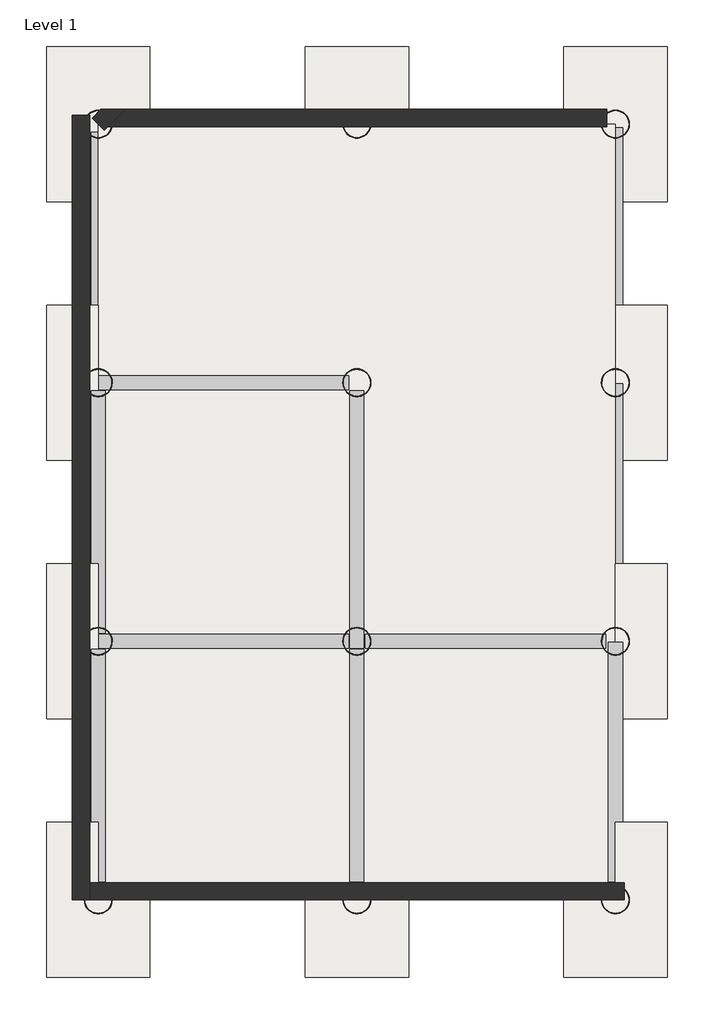
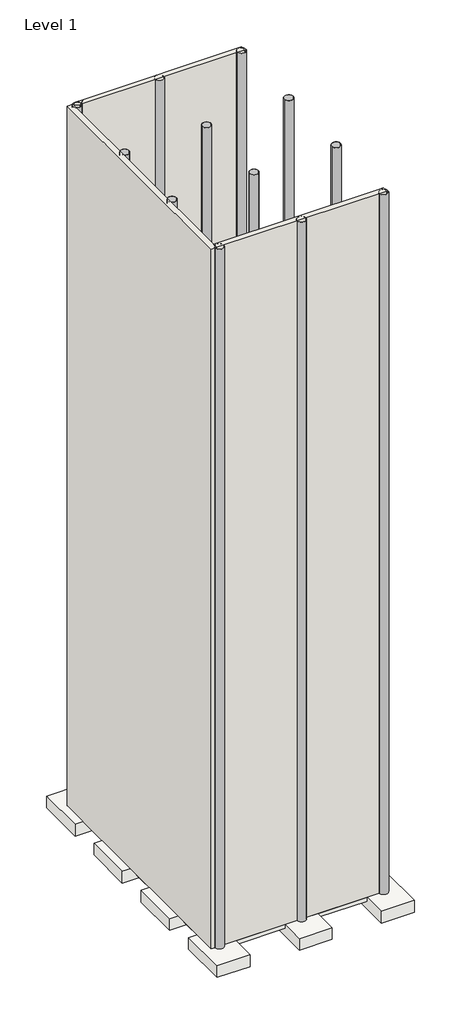
# One storey: 15 beams, 13 slabs, 12 columns, 4 walls.
"""IFC4 building model written with IfcOpenShell, lengths in millimetres."""

from ifc_helpers import new_model, si_unit, frame, origin, place, context, project, spatial, polyline, outline, extrude, faceted_brep, transform, mapped, element, save
from components import ub_universal_beams_ub305x165x40_219eb426, ub_universal_beams_ub305x165x40_d74fc5b0, ub_universal_beams_ub305x165x40_f0dc7efd, ub_universal_beams_ub305x165x40_603755b3, ub_universal_beams_ub305x165x40_59f247e4, ub_universal_beams_ub305x165x40_82a0cad5, ub_universal_beams_ub305x165x40_f6c4464a, ub_universal_beams_ub305x165x40_59e17645, ub_universal_beams_ub305x165x40_3a463868, ub_universal_beams_ub305x165x40_ffb14e35, ub_universal_beams_beam_d94dd637, pipe_column_pipe12std_f9386f83

model = new_model("IFC4")

# Units and contexts
model_context = context("Model", 3, world=origin())
ifc_project = project(units=[si_unit("LENGTHUNIT", "METRE", prefix="MILLI")], contexts=[model_context])

# Site, building, storey
site = spatial("IfcSite", under=ifc_project)
building = spatial("IfcBuilding", under=site)
storey = spatial("IfcBuildingStorey", under=building, Name="Level 1", Elevation=0.0)

# Beams
placement = place(None, origin())
ub_universal_beams_ub305x165x40_shape = ub_universal_beams_ub305x165x40_219eb426(model_context)
element("IfcBeam", 1, ObjectType="UB-Universal Beams : UB305x165x40", at=placement, inside=storey, context=model_context, shape_type="MappedRepresentation", body=[
    mapped(ub_universal_beams_ub305x165x40_shape, transform((13935.1404262, -1814.7314166, -151.7), x_axis=(0.0, 1.0, 0.0), y_axis=(-1.0, 0.0, 0.0), z_axis=(0.0, 0.0, 1.0))),
])
ub_universal_beams_ub305x165x40_2_shape = ub_universal_beams_ub305x165x40_d74fc5b0(model_context)
element("IfcBeam", 2, ObjectType="UB-Universal Beams : UB305x165x40", at=placement, inside=storey, context=model_context, shape_type="MappedRepresentation", body=[
    mapped(ub_universal_beams_ub305x165x40_2_shape, transform((16935.1404262, -1814.7314166, -151.7), x_axis=(0.0, 1.0, 0.0), y_axis=(-1.0, 0.0, 0.0), z_axis=(0.0, 0.0, 1.0))),
])
ub_universal_beams_ub305x165x40_3_shape = ub_universal_beams_ub305x165x40_f0dc7efd(model_context)
element("IfcBeam", 3, ObjectType="UB-Universal Beams : UB305x165x40", at=placement, inside=storey, context=model_context, shape_type="MappedRepresentation", body=[
    mapped(ub_universal_beams_ub305x165x40_3_shape, transform((15435.1404262, -3314.7314166, -151.7), x_axis=(-1.0, 0.0, 0.0), y_axis=(0.0, -1.0, 0.0), z_axis=(0.0, 0.0, 1.0))),
])
element("IfcBeam", 4, ObjectType="UB-Universal Beams : UB305x165x40", at=placement, inside=storey, context=model_context, shape_type="MappedRepresentation", body=[
    mapped(ub_universal_beams_ub305x165x40_3_shape, transform((15435.1404262, -314.7314166, -151.7), x_axis=(-1.0, 0.0, 0.0), y_axis=(0.0, -1.0, 0.0), z_axis=(0.0, 0.0, 1.0))),
])
element("IfcBeam", 5, ObjectType="UB-Universal Beams : UB305x165x40", at=placement, inside=storey, context=model_context, shape_type="MappedRepresentation", body=[
    mapped(ub_universal_beams_ub305x165x40_shape, transform((13935.1404262, 1185.2685834, -151.7), x_axis=(0.0, 1.0, 0.0), y_axis=(-1.0, 0.0, 0.0), z_axis=(0.0, 0.0, 1.0))),
])
ub_universal_beams_ub305x165x40_4_shape = ub_universal_beams_ub305x165x40_603755b3(model_context)
element("IfcBeam", 6, ObjectType="UB-Universal Beams : UB305x165x40", at=placement, inside=storey, context=model_context, shape_type="MappedRepresentation", body=[
    mapped(ub_universal_beams_ub305x165x40_4_shape, transform((15435.1404262, 2685.2685834, -151.7), x_axis=(-1.0, 0.0, 0.0), y_axis=(0.0, -1.0, 0.0), z_axis=(0.0, 0.0, 1.0))),
])
ub_universal_beams_ub305x165x40_5_shape = ub_universal_beams_ub305x165x40_59f247e4(model_context)
element("IfcBeam", 7, ObjectType="UB-Universal Beams : UB305x165x40", at=placement, inside=storey, context=model_context, shape_type="MappedRepresentation", body=[
    mapped(ub_universal_beams_ub305x165x40_5_shape, transform((16935.1404262, 1220.6239224, -151.7), x_axis=(0.0, 1.0, 0.0), y_axis=(-1.0, 0.0, 0.0), z_axis=(0.0, 0.0, 1.0))),
])
ub_universal_beams_ub305x165x40_6_shape = ub_universal_beams_ub305x165x40_82a0cad5(model_context)
element("IfcBeam", 8, ObjectType="UB-Universal Beams : UB305x165x40", at=placement, inside=storey, context=model_context, shape_type="MappedRepresentation", body=[
    mapped(ub_universal_beams_ub305x165x40_6_shape, transform((18435.1404262, -3314.7314166, -151.7), x_axis=(-1.0, 0.0, 0.0), y_axis=(0.0, -1.0, 0.0), z_axis=(0.0, 0.0, 1.0))),
])
element("IfcBeam", 9, ObjectType="UB-Universal Beams : UB305x165x40", at=placement, inside=storey, context=model_context, shape_type="MappedRepresentation", body=[
    mapped(ub_universal_beams_ub305x165x40_6_shape, transform((18435.1404262, -314.7314166, -151.7), x_axis=(-1.0, 0.0, 0.0), y_axis=(0.0, -1.0, 0.0), z_axis=(0.0, 0.0, 1.0))),
])
ub_universal_beams_ub305x165x40_7_shape = ub_universal_beams_ub305x165x40_f6c4464a(model_context)
element("IfcBeam", 10, ObjectType="UB-Universal Beams : UB305x165x40", at=placement, inside=storey, context=model_context, shape_type="MappedRepresentation", body=[
    mapped(ub_universal_beams_ub305x165x40_7_shape, transform((18435.1404262, 2685.2685834, -151.7), x_axis=(-1.0, 0.0, 0.0), y_axis=(0.0, -1.0, 0.0), z_axis=(0.0, 0.0, 1.0))),
])
ub_universal_beams_ub305x165x40_8_shape = ub_universal_beams_ub305x165x40_59e17645(model_context)
element("IfcBeam", 11, ObjectType="UB-Universal Beams : UB305x165x40", at=placement, inside=storey, context=model_context, shape_type="MappedRepresentation", body=[
    mapped(ub_universal_beams_ub305x165x40_8_shape, transform((19935.1404262, -1814.7314166, -151.7), x_axis=(0.0, 1.0, 0.0), y_axis=(-1.0, 0.0, 0.0), z_axis=(0.0, 0.0, 1.0))),
])
ub_universal_beams_ub305x165x40_9_shape = ub_universal_beams_ub305x165x40_3a463868(model_context)
element("IfcBeam", 12, ObjectType="UB-Universal Beams : UB305x165x40", at=placement, inside=storey, context=model_context, shape_type="MappedRepresentation", body=[
    mapped(ub_universal_beams_ub305x165x40_9_shape, transform((19935.1404262, 1220.6239224, -151.7), x_axis=(0.0, 1.0, 0.0), y_axis=(-1.0, 0.0, 0.0), z_axis=(0.0, 0.0, 1.0))),
])
ub_universal_beams_ub305x165x40_10_shape = ub_universal_beams_ub305x165x40_ffb14e35(model_context)
element("IfcBeam", 13, ObjectType="UB-Universal Beams : UB305x165x40", at=placement, inside=storey, context=model_context, shape_type="MappedRepresentation", body=[
    mapped(ub_universal_beams_ub305x165x40_10_shape, transform((13935.1404262, -4764.7314166, -151.7), x_axis=(0.0, 1.0, 0.0), y_axis=(-1.0, 0.0, 0.0), z_axis=(0.0, 0.0, 1.0))),
])
element("IfcBeam", 14, ObjectType="UB-Universal Beams : UB305x165x40", at=placement, inside=storey, context=model_context, shape_type="MappedRepresentation", body=[
    mapped(ub_universal_beams_ub305x165x40_10_shape, transform((16935.1404262, -4764.7314166, -151.7), x_axis=(0.0, 1.0, 0.0), y_axis=(-1.0, 0.0, 0.0), z_axis=(0.0, 0.0, 1.0))),
])
ub_universal_beams_beam_shape = ub_universal_beams_beam_d94dd637(model_context)
element("IfcBeam", 15, ObjectType="UB-Universal Beams : beam", at=placement, inside=storey, context=model_context, shape_type="MappedRepresentation", body=[
    mapped(ub_universal_beams_beam_shape, transform((19935.1404262, -4764.7314166, -151.7), x_axis=(0.0, 1.0, 0.0), y_axis=(-1.0, 0.0, 0.0), z_axis=(0.0, 0.0, 1.0))),
])

# Columns
pipe_column_pipe12std_shape = pipe_column_pipe12std_f9386f83(model_context)
element("IfcColumn", 16, ObjectType="Pipe Column : Pipe12STD", at=placement, inside=storey, context=model_context, shape_type="MappedRepresentation", body=[
    mapped(pipe_column_pipe12std_shape, transform((13935.1404262, -6314.7314166, 0.0), x_axis=(-1.0, 0.0, 0.0), y_axis=(0.0, -1.0, 0.0), z_axis=(0.0, 0.0, 1.0))),
])
element("IfcColumn", 17, ObjectType="Pipe Column : Pipe12STD", at=placement, inside=storey, context=model_context, shape_type="MappedRepresentation", body=[
    mapped(pipe_column_pipe12std_shape, transform((16935.1404262, -6314.7314166, 0.0), x_axis=(-1.0, 0.0, 0.0), y_axis=(0.0, -1.0, 0.0), z_axis=(0.0, 0.0, 1.0))),
])
element("IfcColumn", 18, ObjectType="Pipe Column : Pipe12STD", at=placement, inside=storey, context=model_context, shape_type="MappedRepresentation", body=[
    mapped(pipe_column_pipe12std_shape, transform((19935.1404262, -6314.7314166, 0.0), x_axis=(-1.0, 0.0, 0.0), y_axis=(0.0, -1.0, 0.0), z_axis=(0.0, 0.0, 1.0))),
])
element("IfcColumn", 19, ObjectType="Pipe Column : Pipe12STD", at=placement, inside=storey, context=model_context, shape_type="MappedRepresentation", body=[
    mapped(pipe_column_pipe12std_shape, transform((13935.1404262, -3314.7314166, 0.0), x_axis=(-1.0, 0.0, 0.0), y_axis=(0.0, -1.0, 0.0), z_axis=(0.0, 0.0, 1.0))),
])
element("IfcColumn", 20, ObjectType="Pipe Column : Pipe12STD", at=placement, inside=storey, context=model_context, shape_type="MappedRepresentation", body=[
    mapped(pipe_column_pipe12std_shape, transform((13935.1404262, -314.7314166, 0.0), x_axis=(-1.0, 0.0, 0.0), y_axis=(0.0, -1.0, 0.0), z_axis=(0.0, 0.0, 1.0))),
])
element("IfcColumn", 21, ObjectType="Pipe Column : Pipe12STD", at=placement, inside=storey, context=model_context, shape_type="MappedRepresentation", body=[
    mapped(pipe_column_pipe12std_shape, transform((13935.1404262, 2685.2685834, 0.0), x_axis=(-1.0, 0.0, 0.0), y_axis=(0.0, -1.0, 0.0), z_axis=(0.0, 0.0, 1.0))),
])
element("IfcColumn", 22, ObjectType="Pipe Column : Pipe12STD", at=placement, inside=storey, context=model_context, shape_type="MappedRepresentation", body=[
    mapped(pipe_column_pipe12std_shape, transform((16935.1404262, -3314.7314166, 0.0), x_axis=(-1.0, 0.0, 0.0), y_axis=(0.0, -1.0, 0.0), z_axis=(0.0, 0.0, 1.0))),
])
element("IfcColumn", 23, ObjectType="Pipe Column : Pipe12STD", at=placement, inside=storey, context=model_context, shape_type="MappedRepresentation", body=[
    mapped(pipe_column_pipe12std_shape, transform((19935.1404262, -3314.7314166, 0.0), x_axis=(-1.0, 0.0, 0.0), y_axis=(0.0, -1.0, 0.0), z_axis=(0.0, 0.0, 1.0))),
])
element("IfcColumn", 24, ObjectType="Pipe Column : Pipe12STD", at=placement, inside=storey, context=model_context, shape_type="MappedRepresentation", body=[
    mapped(pipe_column_pipe12std_shape, transform((16935.1404262, -314.7314166, 0.0), x_axis=(-1.0, 0.0, 0.0), y_axis=(0.0, -1.0, 0.0), z_axis=(0.0, 0.0, 1.0))),
])
element("IfcColumn", 25, ObjectType="Pipe Column : Pipe12STD", at=placement, inside=storey, context=model_context, shape_type="MappedRepresentation", body=[
    mapped(pipe_column_pipe12std_shape, transform((19935.1404262, -314.7314166, 0.0), x_axis=(-1.0, 0.0, 0.0), y_axis=(0.0, -1.0, 0.0), z_axis=(0.0, 0.0, 1.0))),
])
element("IfcColumn", 26, ObjectType="Pipe Column : Pipe12STD", at=placement, inside=storey, context=model_context, shape_type="MappedRepresentation", body=[
    mapped(pipe_column_pipe12std_shape, transform((16935.1404262, 2685.2685834, 0.0), x_axis=(-1.0, 0.0, 0.0), y_axis=(0.0, -1.0, 0.0), z_axis=(0.0, 0.0, 1.0))),
])
element("IfcColumn", 27, ObjectType="Pipe Column : Pipe12STD", at=placement, inside=storey, context=model_context, shape_type="MappedRepresentation", body=[
    mapped(pipe_column_pipe12std_shape, transform((19935.1404262, 2685.2685834, 0.0), x_axis=(-1.0, 0.0, 0.0), y_axis=(0.0, -1.0, 0.0), z_axis=(0.0, 0.0, 1.0))),
])

# Slabs
element("IfcSlab", 28, ObjectType="150mm Foundation Slab", at=placement, inside=storey, context=model_context, shape_type="Brep", body=[
    faceted_brep([(13935.1404262, -6314.7314166, -150.0), (13935.1404262, -5414.7314166, -150.0), (13935.1404262, -4214.7314166, -150.0), (13935.1404262, -2414.7314166, -150.0), (13935.1404262, -1214.7314166, -150.0), (13935.1404262, 585.2685834, -150.0), (13935.1404262, 1785.2685834, -150.0), (13935.1404262, 2685.2685834, -150.0), (14535.1404262, 2685.2685834, -150.0), (16335.1404262, 2685.2685834, -150.0), (17535.1404262, 2685.2685834, -150.0), (19335.1404262, 2685.2685834, -150.0), (19935.1404262, 2685.2685834, -150.0), (19935.1404262, 1785.2685834, -150.0), (19935.1404262, 585.2685834, -150.0), (19935.1404262, -1214.7314166, -150.0), (19935.1404262, -2414.7314166, -150.0), (19935.1404262, -4214.7314166, -150.0), (19935.1404262, -5414.7314166, -150.0), (19935.1404262, -6314.7314166, -150.0), (19335.1404262, -6314.7314166, -150.0), (17535.1404262, -6314.7314166, -150.0), (16335.1404262, -6314.7314166, -150.0), (14535.1404262, -6314.7314166, -150.0), (13935.1404262, -6314.7314166, 0.0), (14535.1404262, -6314.7314166, 0.0), (16335.1404262, -6314.7314166, 0.0), (17535.1404262, -6314.7314166, 0.0), (19335.1404262, -6314.7314166, 0.0), (19935.1404262, -6314.7314166, 0.0), (19935.1404262, -5414.7314166, 0.0), (19935.1404262, -4214.7314166, 0.0), (19935.1404262, -2414.7314166, 0.0), (19935.1404262, -1214.7314166, 0.0), (19935.1404262, 585.2685834, 0.0), (19935.1404262, 1785.2685834, 0.0), (19935.1404262, 2685.2685834, 0.0), (19335.1404262, 2685.2685834, 0.0), (17535.1404262, 2685.2685834, 0.0), (16335.1404262, 2685.2685834, 0.0), (14535.1404262, 2685.2685834, 0.0), (13935.1404262, 2685.2685834, 0.0), (13935.1404262, 1785.2685834, 0.0), (13935.1404262, 585.2685834, 0.0), (13935.1404262, -1214.7314166, 0.0), (13935.1404262, -2414.7314166, 0.0), (13935.1404262, -4214.7314166, 0.0), (13935.1404262, -5414.7314166, 0.0)], [[[0, 1, 2, 3, 4, 5, 6, 7, 8, 9, 10, 11, 12, 13, 14, 15, 16, 17, 18, 19, 20, 21, 22, 23]], [[24, 25, 26, 27, 28, 29, 30, 31, 32, 33, 34, 35, 36, 37, 38, 39, 40, 41, 42, 43, 44, 45, 46, 47]], [[7, 6, 5, 4, 3, 2, 1, 0, 24, 47, 46, 45, 44, 43, 42, 41]], [[12, 11, 10, 9, 8, 7, 41, 40, 39, 38, 37, 36]], [[19, 18, 17, 16, 15, 14, 13, 12, 36, 35, 34, 33, 32, 31, 30, 29]], [[0, 23, 22, 21, 20, 19, 29, 28, 27, 26, 25, 24]]]),
])
element("IfcSlab", 29, ObjectType="M_Footing-Rectangular : 1800 x 1200 x 450mm", at=placement, inside=storey, context=model_context, shape_type="Brep", body=[
    faceted_brep([(13335.1404262, -7214.7314166, 0.0), (14535.1404262, -7214.7314166, 0.0), (14535.1404262, -6314.7314166, 0.0), (13935.1404262, -6314.7314166, 0.0), (13935.1404262, -5414.7314166, 0.0), (13335.1404262, -5414.7314166, 0.0), (13335.1404262, -7214.7314166, -450.0), (13335.1404262, -5414.7314166, -450.0), (14535.1404262, -5414.7314166, -450.0), (14535.1404262, -7214.7314166, -450.0), (14535.1404262, -5414.7314166, -150.0), (14535.1404262, -6314.7314166, -150.0), (13935.1404262, -5414.7314166, -150.0), (13935.1404262, -6314.7314166, -150.0)], [[[0, 1, 2, 3, 4, 5]], [[6, 7, 8, 9]], [[1, 0, 6, 9]], [[9, 8, 10, 11, 2, 1]], [[8, 7, 5, 4, 12, 10]], [[0, 5, 7, 6]], [[13, 11, 10, 12]], [[3, 13, 12, 4]], [[13, 3, 2, 11]]]),
])
element("IfcSlab", 30, ObjectType="M_Footing-Rectangular : 1800 x 1200 x 450mm", at=placement, inside=storey, context=model_context, shape_type="SweptSolid", body=[
    extrude(outline(polyline([(-5414.7314166, -450.0), (-7214.7314166, -450.0), (-7214.7314166, 0.0), (-6314.7314166, 0.0), (-6314.7314166, -150.0), (-5414.7314166, -150.0), (-5414.7314166, -450.0)])), frame((16335.1404262, 0.0, 0.0), z_axis=(1.0, 0.0, 0.0), x_axis=(0.0, 1.0, 0.0)), (0.0, 0.0, 1.0), 1200.0),
])
element("IfcSlab", 31, ObjectType="M_Footing-Rectangular : 1800 x 1200 x 450mm", at=placement, inside=storey, context=model_context, shape_type="Brep", body=[
    faceted_brep([(19335.1404262, -7214.7314166, 0.0), (20535.1404262, -7214.7314166, 0.0), (20535.1404262, -5414.7314166, 0.0), (19935.1404262, -5414.7314166, 0.0), (19935.1404262, -6314.7314166, 0.0), (19335.1404262, -6314.7314166, 0.0), (19335.1404262, -7214.7314166, -450.0), (19335.1404262, -5414.7314166, -450.0), (20535.1404262, -5414.7314166, -450.0), (20535.1404262, -7214.7314166, -450.0), (19335.1404262, -5414.7314166, -150.0), (19935.1404262, -5414.7314166, -150.0), (19335.1404262, -6314.7314166, -150.0), (19935.1404262, -6314.7314166, -150.0)], [[[0, 1, 2, 3, 4, 5]], [[6, 7, 8, 9]], [[1, 0, 6, 9]], [[2, 1, 9, 8]], [[8, 7, 10, 11, 3, 2]], [[7, 6, 0, 5, 12, 10]], [[12, 13, 11, 10]], [[13, 4, 3, 11]], [[4, 13, 12, 5]]]),
])
element("IfcSlab", 32, ObjectType="M_Footing-Rectangular : 1800 x 1200 x 450mm", at=placement, inside=storey, context=model_context, shape_type="SweptSolid", body=[
    extrude(outline(polyline([(-450.0, 13335.1404262), (-450.0, 14535.1404262), (-150.0, 14535.1404262), (-150.0, 13935.1404262), (0.0, 13935.1404262), (0.0, 13335.1404262), (-450.0, 13335.1404262)])), frame((0.0, -4214.7314166, 0.0), z_axis=(0.0, 1.0, 0.0), x_axis=(0.0, 0.0, 1.0)), (0.0, 0.0, 1.0), 1800.0),
])
element("IfcSlab", 33, ObjectType="M_Footing-Rectangular : 1800 x 1200 x 450mm", at=placement, inside=storey, context=model_context, shape_type="SweptSolid", body=[
    extrude(outline(polyline([(-450.0, 13335.1404262), (-450.0, 14535.1404262), (-150.0, 14535.1404262), (-150.0, 13935.1404262), (0.0, 13935.1404262), (0.0, 13335.1404262), (-450.0, 13335.1404262)])), frame((0.0, -1214.7314166, 0.0), z_axis=(0.0, 1.0, 0.0), x_axis=(0.0, 0.0, 1.0)), (0.0, 0.0, 1.0), 1800.0),
])
element("IfcSlab", 34, ObjectType="M_Footing-Rectangular : 1800 x 1200 x 450mm", at=placement, inside=storey, context=model_context, shape_type="Brep", body=[
    faceted_brep([(14535.1404262, 3585.2685834, 0.0), (13335.1404262, 3585.2685834, 0.0), (13335.1404262, 1785.2685834, 0.0), (13935.1404262, 1785.2685834, 0.0), (13935.1404262, 2685.2685834, 0.0), (14535.1404262, 2685.2685834, 0.0), (13335.1404262, 1785.2685834, -450.0), (13335.1404262, 3585.2685834, -450.0), (14535.1404262, 3585.2685834, -450.0), (14535.1404262, 1785.2685834, -450.0), (14535.1404262, 1785.2685834, -150.0), (13935.1404262, 1785.2685834, -150.0), (14535.1404262, 2685.2685834, -150.0), (13935.1404262, 2685.2685834, -150.0)], [[[0, 1, 2, 3, 4, 5]], [[6, 7, 8, 9]], [[6, 9, 10, 11, 3, 2]], [[9, 8, 0, 5, 12, 10]], [[1, 0, 8, 7]], [[2, 1, 7, 6]], [[12, 13, 11, 10]], [[13, 4, 3, 11]], [[4, 13, 12, 5]]]),
])
element("IfcSlab", 35, ObjectType="M_Footing-Rectangular : 1800 x 1200 x 450mm", at=placement, inside=storey, context=model_context, shape_type="SweptSolid", body=[
    extrude(outline(polyline([(16335.1404262, -4214.7314166), (16335.1404262, -2414.7314166), (17535.1404262, -2414.7314166), (17535.1404262, -4214.7314166), (16335.1404262, -4214.7314166)])), frame((0.0, 0.0, -450.0), z_axis=(0.0, 0.0, 1.0), x_axis=(1.0, 0.0, 0.0)), (0.0, 0.0, 1.0), 300.0),
])
element("IfcSlab", 36, ObjectType="M_Footing-Rectangular : 1800 x 1200 x 450mm", at=placement, inside=storey, context=model_context, shape_type="SweptSolid", body=[
    extrude(outline(polyline([(-450.0, 19335.1404262), (-450.0, 20535.1404262), (0.0, 20535.1404262), (0.0, 19935.1404262), (-150.0, 19935.1404262), (-150.0, 19335.1404262), (-450.0, 19335.1404262)])), frame((0.0, -4214.7314166, 0.0), z_axis=(0.0, 1.0, 0.0), x_axis=(0.0, 0.0, 1.0)), (0.0, 0.0, 1.0), 1800.0),
])
element("IfcSlab", 37, ObjectType="M_Footing-Rectangular : 1800 x 1200 x 450mm", at=placement, inside=storey, context=model_context, shape_type="SweptSolid", body=[
    extrude(outline(polyline([(16335.1404262, -1214.7314166), (16335.1404262, 585.2685834), (17535.1404262, 585.2685834), (17535.1404262, -1214.7314166), (16335.1404262, -1214.7314166)])), frame((0.0, 0.0, -450.0), z_axis=(0.0, 0.0, 1.0), x_axis=(1.0, 0.0, 0.0)), (0.0, 0.0, 1.0), 300.0),
])
element("IfcSlab", 38, ObjectType="M_Footing-Rectangular : 1800 x 1200 x 450mm", at=placement, inside=storey, context=model_context, shape_type="SweptSolid", body=[
    extrude(outline(polyline([(-450.0, 19335.1404262), (-450.0, 20535.1404262), (0.0, 20535.1404262), (0.0, 19935.1404262), (-150.0, 19935.1404262), (-150.0, 19335.1404262), (-450.0, 19335.1404262)])), frame((0.0, -1214.7314166, 0.0), z_axis=(0.0, 1.0, 0.0), x_axis=(0.0, 0.0, 1.0)), (0.0, 0.0, 1.0), 1800.0),
])
element("IfcSlab", 39, ObjectType="M_Footing-Rectangular : 1800 x 1200 x 450mm", at=placement, inside=storey, context=model_context, shape_type="SweptSolid", body=[
    extrude(outline(polyline([(3585.2685834, -450.0), (1785.2685834, -450.0), (1785.2685834, -150.0), (2685.2685834, -150.0), (2685.2685834, 0.0), (3585.2685834, 0.0), (3585.2685834, -450.0)])), frame((16335.1404262, 0.0, 0.0), z_axis=(1.0, 0.0, 0.0), x_axis=(0.0, 1.0, 0.0)), (0.0, 0.0, 1.0), 1200.0),
])
element("IfcSlab", 40, ObjectType="M_Footing-Rectangular : 1800 x 1200 x 450mm", at=placement, inside=storey, context=model_context, shape_type="Brep", body=[
    faceted_brep([(20535.1404262, 1785.2685834, 0.0), (20535.1404262, 3585.2685834, 0.0), (19335.1404262, 3585.2685834, 0.0), (19335.1404262, 2685.2685834, 0.0), (19935.1404262, 2685.2685834, 0.0), (19935.1404262, 1785.2685834, 0.0), (19335.1404262, 1785.2685834, -450.0), (19335.1404262, 3585.2685834, -450.0), (20535.1404262, 3585.2685834, -450.0), (20535.1404262, 1785.2685834, -450.0), (19935.1404262, 1785.2685834, -150.0), (19335.1404262, 1785.2685834, -150.0), (19335.1404262, 2685.2685834, -150.0), (19935.1404262, 2685.2685834, -150.0)], [[[0, 1, 2, 3, 4, 5]], [[6, 7, 8, 9]], [[6, 9, 0, 5, 10, 11]], [[1, 0, 9, 8]], [[2, 1, 8, 7]], [[7, 6, 11, 12, 3, 2]], [[10, 13, 12, 11]], [[13, 4, 3, 12]], [[4, 13, 10, 5]]]),
])

# Walls
element("IfcWall", 41, ObjectType="Generic - 200mm", at=placement, inside=storey, context=model_context, shape_type="Brep", body=[
    faceted_brep([(14005.8511043, 2614.5579052, 0.0), (14047.2724606, 2655.9792615, 0.0), (14247.2724606, 2855.9792615, 0.0), (14247.2724606, 2855.9792615, 27000.0), (14047.2724606, 2655.9792615, 27000.0), (14005.8511043, 2614.5579052, 27000.0), (13864.4297481, 2755.9792615, 0.0), (13864.4297481, 2755.9792615, 27000.0), (13964.4297481, 2855.9792615, 27000.0), (13964.4297481, 2855.9792615, 0.0)], [[[0, 1, 2, 3, 4, 5]], [[6, 7, 8, 9]], [[2, 1, 0, 6, 9]], [[5, 4, 3, 8, 7]], [[0, 5, 7, 6]], [[3, 2, 9, 8]]]),
])
element("IfcWall", 42, ObjectType="Generic - 200mm", at=placement, inside=storey, context=model_context, shape_type="Brep", body=[
    faceted_brep([(14047.2724606, 2655.9792615, 0.0), (19835.1404262, 2655.9792615, 0.0), (19835.1404262, 2655.9792615, 3000.0), (20035.1404262, 2655.9792615, 3000.0), (20035.1404262, 2655.9792615, 6000.0), (20035.1404262, 2655.9792615, 9000.0), (20035.1404262, 2655.9792615, 12000.0), (20035.1404262, 2655.9792615, 15000.0), (20035.1404262, 2655.9792615, 18000.0), (20035.1404262, 2655.9792615, 21000.0), (20035.1404262, 2655.9792615, 24000.0), (20035.1404262, 2655.9792615, 27000.0), (19835.1404262, 2655.9792615, 27000.0), (14047.2724606, 2655.9792615, 27000.0), (14247.2724606, 2855.9792615, 0.0), (14247.2724606, 2855.9792615, 27000.0), (20035.1404262, 2855.9792615, 27000.0), (20035.1404262, 2855.9792615, 3000.0), (19835.1404262, 2855.9792615, 3000.0), (19835.1404262, 2855.9792615, 0.0)], [[[0, 1, 2, 3, 4, 5, 6, 7, 8, 9, 10, 11, 12, 13]], [[14, 15, 16, 17, 18, 19]], [[1, 0, 14, 19]], [[13, 12, 11, 16, 15]], [[17, 3, 2, 18]], [[2, 1, 19, 18]], [[3, 17, 16, 11, 10, 9, 8, 7, 6, 5, 4]], [[0, 13, 15, 14]]]),
])
element("IfcWall", 43, ObjectType="Generic - 200mm", at=placement, inside=storey, context=model_context, shape_type="Brep", body=[
    faceted_brep([(20035.1404262, -6114.7314166, 27000.0), (20035.1404262, -6114.7314166, 24000.0), (20035.1404262, -6114.7314166, 21000.0), (20035.1404262, -6114.7314166, 18000.0), (20035.1404262, -6114.7314166, 15000.0), (20035.1404262, -6114.7314166, 12000.0), (20035.1404262, -6114.7314166, 9000.0), (20035.1404262, -6114.7314166, 6000.0), (20035.1404262, -6114.7314166, 3000.0), (20035.1404262, -6114.7314166, 0.0), (19835.1404262, -6114.7314166, 0.0), (13835.1404262, -6114.7314166, 0.0), (13835.1404262, -6114.7314166, 27000.0), (19835.1404262, -6114.7314166, 27000.0), (20035.1404262, -6314.7314166, 0.0), (20035.1404262, -6314.7314166, 27000.0), (13835.1404262, -6314.7314166, 27000.0), (13835.1404262, -6314.7314166, 0.0)], [[[0, 1, 2, 3, 4, 5, 6, 7, 8, 9, 10, 11, 12, 13]], [[14, 15, 16, 17]], [[11, 10, 9, 14, 17]], [[0, 13, 12, 16, 15]], [[0, 15, 14, 9, 8, 7, 6, 5, 4, 3, 2, 1]], [[12, 11, 17, 16]]]),
])
element("IfcWall", 44, ObjectType="Generic - 200mm", at=placement, inside=storey, context=model_context, shape_type="Brep", body=[
    faceted_brep([(13835.1404262, -6314.7314166, 0.0), (13835.1404262, -6114.7314166, 0.0), (13835.1404262, 2785.2685834, 0.0), (13835.1404262, 2785.2685834, 27000.0), (13835.1404262, -6114.7314166, 27000.0), (13835.1404262, -6314.7314166, 27000.0), (13635.1404262, -6314.7314166, 0.0), (13635.1404262, -6314.7314166, 27000.0), (13635.1404262, 2785.2685834, 27000.0), (13635.1404262, 2785.2685834, 0.0)], [[[0, 1, 2, 3, 4, 5]], [[6, 7, 8, 9]], [[2, 1, 0, 6, 9]], [[3, 2, 9, 8]], [[5, 4, 3, 8, 7]], [[0, 5, 7, 6]]]),
])

save(model, "model.ifc")

# Revit data of these elements
# Grids (mm)
#   "1": line (7751.128, -6314.731) -> (24761.391, -6314.731)
#   "2": line (13935.14, 6118.893) -> (13935.14, -6314.731)
#   "3": line (7751.128, -3314.731) -> (24761.391, -3314.731)
#   "4": line (7751.128, -314.731) -> (24761.391, -314.731)
#   "5": line (7751.128, 2685.269) -> (24761.391, 2685.269)
#   "6": line (16935.14, 6118.893) -> (16935.14, -6314.731)
#   "7": line (19935.14, 6118.893) -> (19935.14, -6314.731)
#   "8": line (7751.128, -6314.731) -> (24761.391, -6314.731)
#   "9": line (7751.128, -3314.731) -> (24761.391, -3314.731)
#   "10": line (7751.128, -314.731) -> (24761.391, -314.731)
#   "11": line (7751.128, 2685.269) -> (24761.391, 2685.269)
#   "12": line (7751.128, -6314.731) -> (24761.391, -6314.731)
#   "13": line (7751.128, -3314.731) -> (24761.391, -3314.731)
#   "14": line (7751.128, -314.731) -> (24761.391, -314.731)
#   "15": line (7751.128, 2685.269) -> (24761.391, 2685.269)
#   "16": line (7751.128, -6314.731) -> (24761.391, -6314.731)
#   "17": line (7751.128, -3314.731) -> (24761.391, -3314.731)
#   "18": line (7751.128, -314.731) -> (24761.391, -314.731)
#   "19": line (7751.128, 2685.269) -> (24761.391, 2685.269)
#   "20": line (7751.128, -6314.731) -> (24761.391, -6314.731)
#   "21": line (7751.128, -3314.731) -> (24761.391, -3314.731)
#   "22": line (7751.128, -314.731) -> (24761.391, -314.731)
#   "23": line (7751.128, 2685.269) -> (24761.391, 2685.269)
#   "24": line (7751.128, -6314.731) -> (24761.391, -6314.731)
#   "25": line (7751.128, -3314.731) -> (24761.391, -3314.731)
#   "26": line (7751.128, -314.731) -> (24761.391, -314.731)
#   "27": line (7751.128, 2685.269) -> (24761.391, 2685.269)
#   "28": line (7751.128, -6314.731) -> (24761.391, -6314.731)
#   "29": line (7751.128, -3314.731) -> (24761.391, -3314.731)
#   "30": line (7751.128, -314.731) -> (24761.391, -314.731)
#   "31": line (7751.128, 2685.269) -> (24761.391, 2685.269)
#   "32": line (7751.128, -6314.731) -> (24761.391, -6314.731)
#   "33": line (7751.128, -3314.731) -> (24761.391, -3314.731)
#   "34": line (7751.128, -314.731) -> (24761.391, -314.731)
#   "35": line (7751.128, 2685.269) -> (24761.391, 2685.269)
#   "36": line (7751.128, -6314.731) -> (24761.391, -6314.731)
#   "37": line (7751.128, -3314.731) -> (24761.391, -3314.731)
#   "38": line (7751.128, -314.731) -> (24761.391, -314.731)
#   "39": line (7751.128, 2685.269) -> (24761.391, 2685.269)
#   "40": line (7751.128, -6314.731) -> (24761.391, -6314.731)
#   "41": line (7751.128, -3314.731) -> (24761.391, -3314.731)
#   "42": line (7751.128, -314.731) -> (24761.391, -314.731)
#   "43": line (7751.128, 2685.269) -> (24761.391, 2685.269)
# Type "UB-Universal Beams : UB305x165x40"
#   Section Name Key = "UB305X165X40"
#   Width = 16.5 cm
#   Web Thickness = 0.6 cm
#   Web Fillet = 0.89 cm
#   Warping Constant = 164000.0 cm⁶
#   Torsional Moment of Inertia = 14.70 cm⁴
#   Section Area = 51.3 cm²
#   Plastic Modulus weak axis = 142.0 cm³
#   Plastic Modulus strong axis = 623.0 cm³
#   Nominal Weight = 40.2999 kgf/m
#   Moment of Inertia weak axis = 764.00 cm⁴
#   Moment of Inertia strong axis = 8503.00 cm⁴
#   Height = 30.34 cm
#   Flange Thickness = 1.02 cm
#   Elastic Modulus weak axis = 92.6 cm³
#   Elastic Modulus strong axis = 560.0 cm³
#   Centroid Vertical = 15.17 cm
#   Centroid Horizontal = 8.25 cm
#   Bolt Spacing = 9.0 cm
#   Length [instance default] = 1.5 m
#   Structural Material [instance default] = Metal - Steel 43-275
#   Type Comments = ""
#   Assembly Code = ""
# Type "UB-Universal Beams : beam"
#   Section Name Key = "UB305X165X40"
#   Width = 16.5 cm
#   Web Thickness = 0.6 cm
#   Web Fillet = 0.89 cm
#   Warping Constant = 164000.0 cm⁶
#   Torsional Moment of Inertia = 14.70 cm⁴
#   Section Area = 51.3 cm²
#   Plastic Modulus weak axis = 142.0 cm³
#   Plastic Modulus strong axis = 623.0 cm³
#   Nominal Weight = 40.2999 kgf/m
#   Moment of Inertia weak axis = 764.00 cm⁴
#   Moment of Inertia strong axis = 8503.00 cm⁴
#   Height = 30.34 cm
#   Flange Thickness = 1.02 cm
#   Elastic Modulus weak axis = 92.6 cm³
#   Elastic Modulus strong axis = 560.0 cm³
#   Centroid Vertical = 15.17 cm
#   Centroid Horizontal = 8.25 cm
#   Bolt Spacing = 9.0 cm
#   Length [instance default] = 1.5 m
#   Structural Material [instance default] = Metal - Steel 43-275
#   Type Comments = ""
#   Assembly Code = ""
# Type "Pipe Column : Pipe12STD"
#   Section Name Key = "Pipe 12 Std"
#   Assembly Code = "B10"
#   Wall Nominal Thickness = 0.9525 cm
#   Wall Design Thickness = 0.8865 cm
#   Torsional Moment of Inertia = 21768.90 cm⁴
#   Section Area = 88.3869 cm²
#   Plastic Modulus weak axis = 879.985 cm³
#   Plastic Modulus strong axis = 879.985 cm³
#   Nominal Weight = 73.8129 kgf/m
#   Moment of Inertia weak axis = 10905.26 cm⁴
#   Moment of Inertia strong axis = 10905.26 cm⁴
#   Elastic Modulus weak axis = 671.87 cm³
#   Elastic Modulus strong axis = 671.87 cm³
#   Diameter = 32.512 cm
#   Centroid Vertical = 16.256 cm
#   Centroid Horizontal = 16.256 cm
#   Structural Material [instance default] = Steel ASTM A53
#   Warping Constant = (empty or 0)
#   Torsional Modulus = 0
#   Principal Axes Angle = 0
# Type "150mm Foundation Slab"
#   Layers, outside or top first: 0.15 m "Concrete, Cast-in-Place gray" (function 1)
# Type "M_Footing-Rectangular : 1800 x 1200 x 450mm"
#   Width = 1.2 m
#   Length = 1.8 m
#   Foundation Thickness = 0.45 m
#   Structural Material [instance default] = Concrete, Cast-in-Place gray
#   Assembly Code = ""
# Type "Generic - 200mm"
#   Layers, outside or top first: 0.2 m no material (function 1)
# Elements 1, 2, 3, 4, 5, 6, 7, 8, 9, 10, 11, 12, 13, 14 (IfcBeam, "UB-Universal Beams : UB305x165x40")
#   Structural Material = Metal - Steel 43-275
#   Phase Created = New Construction
#   Materials on its faces: "Metal - Steel 43-275"
# Element 15 (IfcBeam, "UB-Universal Beams : beam")
#   Structural Material = Metal - Steel 43-275
#   Phase Created = New Construction
#   Materials on its faces: "Metal - Steel 43-275"
# Elements 16, 17, 18, 19, 20, 21, 22, 23, 24, 25, 26, 27 (IfcColumn, "Pipe Column : Pipe12STD")
#   Structural Material = Steel ASTM A53
#   Phase Created = New Construction
#   Materials on its faces: "Steel ASTM A53"
# Element 28 (IfcSlab, "150mm Foundation Slab")
#   built-in parameter 1001955 = 3.14159 (stored number, unit not read)
#   Height Offset From Level = 0 m
#   built-in parameter 1001954 = 1
#   Phase Created = New Construction
#   Materials on its faces: "Concrete, Cast-in-Place gray"
# Elements 29, 30, 31, 32, 33, 34, 35, 36, 37, 38, 39, 40 (IfcSlab, "M_Footing-Rectangular : 1800 x 1200 x 450mm")
#   Comments = ""
#   Structural Material = Concrete, Cast-in-Place gray
#   Phase Created = New Construction
#   Materials on its faces: "Concrete, Cast-in-Place gray"
# Elements 41, 42 (IfcWall, "Generic - 200mm")
#   Top Offset = 0 m
#   Base Offset = 0 m
#   wall height = 27 m
#   Phase Created = New Construction
#   Base Constraint = Level 1
#   Top Constraint = Level 10
#   Materials on its faces: "Default Wall"
# Elements 43, 44 (IfcWall, "Generic - 200mm")
#   Comments = ""
#   Top Offset = 0 m
#   Base Offset = 0 m
#   wall height = 27 m
#   Phase Created = New Construction
#   Base Constraint = Level 1
#   Top Constraint = Level 10
#   Materials on its faces: "Default Wall"
# Materials
#   "Metal - Steel 43-275": class "Metal", colour RGB 247 247 247, transparency 0, Cost = 0
#   "Steel ASTM A53": class "Metal", colour RGB 199 199 199, transparency 0, Description = "Carbon steel", Cost = 0
#   "Concrete, Cast-in-Place gray": class "Concrete", colour RGB 192 192 192, transparency 0, Description = "Cast-in-place concrete", Cost = 0
#   "Default Wall": colour RGB 128 128 128, transparency 0, Cost = 0
